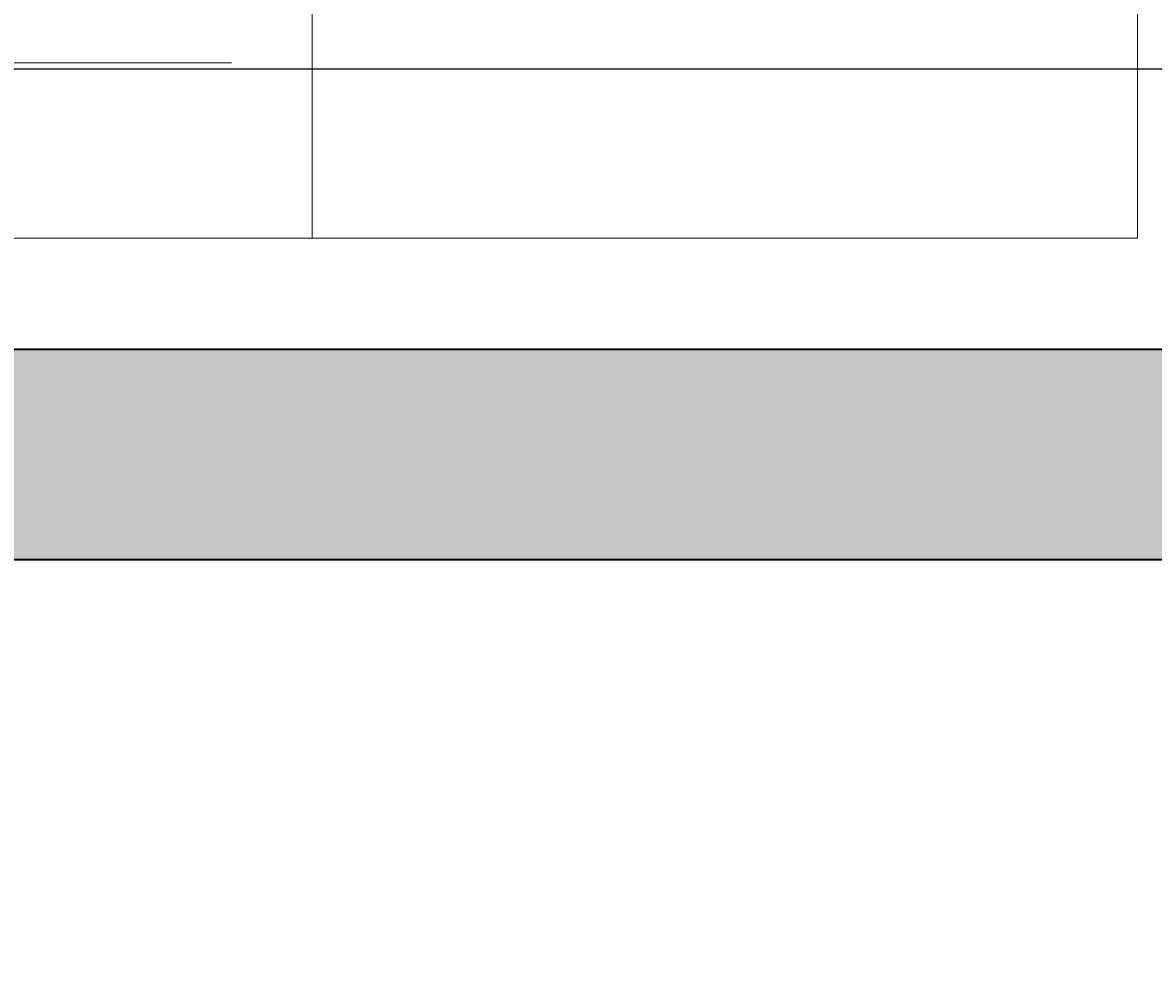
# Model space of a CAD drawing. Units: inches. Extents: x 1998 to 2588, y 1139 to 1977.
# Tile 16 of 134: x 2171 to 2195, y 1576 to 1596. Entities that reach past the tile are written whole.
import ezdxf

# ---------------------------------------------------------------- set-up
doc = ezdxf.new("R2010")
doc.units = ezdxf.units.IN
for name, color, linetype, lineweight in [('A-ANNO-DIMS', 2, 'Continuous', 18), ('A-FLOR-FIXT', 9, 'Continuous', 18), ('A-WALL-PATT', 252, 'Continuous', 13), ('WALL', 200, 'Continuous', 35)]:
    doc.layers.add(name, color=color, linetype=linetype, lineweight=lineweight)
doc.styles.get("Standard").update_dxf_attribs({"font": 'arial.ttf'})
doc.dimstyles.get("Standard").update_dxf_attribs({"dimtxt": 0.18, "dimasz": 0.18, "dimexe": 0.18, "dimexo": 0.0625, "dimgap": 0.09, "dimtad": 0, "dimtih": 1, "dimtoh": 1, "dimdec": 4, "dimzin": 0, "dimdsep": 46, "dimtxsty": 'Standard', "dimcen": 0.09, "dimadec": 0, "dimazin": 0, "dimtfac": 1, "dimtdec": 4, "dimtofl": 0, "dimtmove": 0, "dimatfit": 3, "dimfxl": 1, "dimtolj": 1, "dimtzin": 0, "dimarcsym": 0})

# ---------------------------------------------------------------- blocks, each defined once
blk = doc.blocks.new('SINK-WITH-DRAINBOARD')
for p, q in [((17.653, 0), (17.653, 19.174)), ((15.925, 17.391), (2.574, 17.391)), ((15.925, 15.023), (2.574, 15.023)), ((15.925, 12.848), (2.574, 12.848)), ((15.925, 10.383), (2.574, 10.383)), ((15.925, 8.143), (2.574, 8.143)), ((15.925, 5.899), (2.574, 5.899)), ((15.925, 3.752), (2.574, 3.752))]:
    blk.add_line(p, q)
blk.add_lwpolyline([(35.306, 19.174), (0, 19.174), (0, 0), (35.306, 0)], close=True)
blk.add_circle((25.956, 9.71), 1.353)
blk = doc.blocks.new('*D30')
at = {"layer": 'A-ANNO-DIMS', "color": 0, "lineweight": -2, "transparency": 16777216}
for p, q in [((2407.91, 1636.732), (1997.843, 1636.732)), ((1998.023, 1636.552), (1998.023, 1615.913)), ((1998.023, 1594.912), (1998.023, 1615.552)), ((2407.91, 1594.732), (1997.843, 1594.732))]:
    blk.add_line(p, q, dxfattribs=at)
at = {"layer": 'A-ANNO-DIMS', "color": 0, "transparency": 16777216}
for points in [[(1997.993, 1636.552), (1998.053, 1636.552), (1998.023, 1636.732)], [(1997.993, 1594.912), (1998.053, 1594.912), (1998.023, 1594.732)]]:
    blk.add_solid(points, dxfattribs=at)
at = {"layer": 'Defpoints', "color": 0, "transparency": 16777216}
for p in [(1998.023, 1636.732), (2407.973, 1636.732), (2407.973, 1594.732)]:
    blk.add_point(p, dxfattribs=at)
at = {"layer": 'A-ANNO-DIMS', "color": 0, "transparency": 16777216, "insert": (1998.023, 1615.732), "char_height": 0.18, "attachment_point": 5}
blk.add_mtext('\\A1;42', dxfattribs=at)
blk = doc.blocks.new('*D34')
at = {"layer": 'A-ANNO-DIMS', "color": 0, "lineweight": -2, "transparency": 16777216}
for p, q in [((2407.91, 1594.732), (1997.843, 1594.732)), ((1998.023, 1594.552), (1998.023, 1558.913)), ((1998.023, 1522.912), (1998.023, 1558.552)), ((2407.91, 1522.732), (1997.843, 1522.732))]:
    blk.add_line(p, q, dxfattribs=at)
at = {"layer": 'A-ANNO-DIMS', "color": 0, "transparency": 16777216}
for points in [[(1997.993, 1594.552), (1998.053, 1594.552), (1998.023, 1594.732)], [(1997.993, 1522.912), (1998.053, 1522.912), (1998.023, 1522.732)]]:
    blk.add_solid(points, dxfattribs=at)
at = {"layer": 'Defpoints', "color": 0, "transparency": 16777216}
for p in [(1998.023, 1594.732), (2407.973, 1594.732), (2407.973, 1522.732)]:
    blk.add_point(p, dxfattribs=at)
at = {"layer": 'A-ANNO-DIMS', "color": 0, "transparency": 16777216, "insert": (1998.023, 1558.732), "char_height": 0.18, "attachment_point": 5}
blk.add_mtext('\\A1;72', dxfattribs=at)

msp = doc.modelspace()

# ---------------------------------------------------------------- hatches: boundary and pattern name
at = {"layer": 'A-WALL-PATT'}
h = msp.add_hatch(color=256, dxfattribs=at)
h.dxf.hatch_style = 1
h.paths.add_polyline_path([(2222.9729, 1888.7324), (2099.4125, 1888.7324), (2099.4125, 1879.7324), (2222.9729, 1879.7324)])
h.paths.add_polyline_path([(2096.9729, 1868.3278), (2087.9729, 1868.3278), (2087.9729, 1775.637), (2096.9729, 1775.637)])
h.paths.add_polyline_path([(2227.4729, 1868.3278), (2222.9729, 1868.3278), (2222.9729, 1774.3318), (2227.4729, 1774.3318)])
h.paths.add_polyline_path([(2188.3019, 1759.7324), (2138.6074, 1759.7324), (2099.4125, 1759.7324), (2099.4125, 1755.2324), (2176.9729, 1755.2324), (2188.3019, 1755.2324)])
h.paths.add_polyline_path([(2087.9729, 1759.7324), (2059.4729, 1759.7324), (2059.4729, 1702.7324), (2087.9729, 1702.7324), (2087.9729, 1707.2324), (2063.9729, 1707.2324), (2063.9729, 1755.2324), (2087.9729, 1755.2324)])
h.paths.add_polyline_path([(2096.9729, 1755.2324), (2087.9729, 1755.2324), (2087.9729, 1707.2324), (2096.9729, 1707.2324)])
h.paths.add_polyline_path([(2187.0461, 1707.2324), (2105.9729, 1707.2324), (2096.9729, 1707.2324), (2087.9729, 1707.2324), (2087.9729, 1702.7324), (2105.9729, 1702.7324), (2114.9729, 1702.7324), (2187.0461, 1702.7324)])
h.paths.add_polyline_path([(2181.4729, 1719.2028), (2176.9729, 1719.2028), (2176.9729, 1707.2324), (2181.4729, 1707.2324)])
h.paths.add_polyline_path([(2216.0332, 1588.7324), (2114.9729, 1588.7324), (2105.9729, 1588.7324), (2105.9729, 1584.2324), (2216.0332, 1584.2324)])
h.paths.add_polyline_path([(2077.691, 1588.7324), (2061.4729, 1588.7324), (2061.4729, 1584.2324), (2077.691, 1584.2324)])
h.paths.add_polyline_path([(2105.9729, 1588.7324), (2098.0956, 1588.7324), (2098.0956, 1584.2324), (2105.9729, 1584.2324)])
h.paths.add_polyline_path([(2114.9729, 1596.2642), (2110.1012, 1596.2642), (2105.9729, 1596.2642), (2105.9729, 1588.7324), (2114.9729, 1588.7324)])
h.paths.add_polyline_path([(2114.9729, 1584.2324), (2105.9729, 1584.2324), (2105.9729, 1580.249), (2110.1012, 1580.249), (2114.9729, 1580.249)])
h.paths.add_polyline_path([(2114.9729, 1547.7716), (2110.1012, 1547.7716, -0.0318759), (2105.9729, 1548.035), (2105.9729, 1470.2324), (2108.3775, 1470.2324), (2108.3775, 1465.7324), (2186.2943, 1465.7324), (2186.2943, 1470.2324), (2114.9729, 1470.2324)])
h.paths.add_polyline_path([(2227.4729, 1584.2324), (2222.9729, 1584.2324), (2222.9729, 1486.137), (2227.4729, 1486.137)])
h.paths.add_polyline_path([(2295.4138, 1593.2324), (2227.4729, 1593.2324), (2227.4729, 1588.7324), (2295.4138, 1588.7324), (2295.4138, 1591.8729)])
h.paths.add_polyline_path([(2345.9729, 1627.1165), (2341.4729, 1627.1165), (2341.4729, 1593.2324), (2337.2869, 1593.2324), (2337.2869, 1591.8729), (2337.2869, 1588.7324), (2345.9729, 1588.7324)])
h.paths.add_polyline_path([(2291.9729, 1588.7324), (2287.4729, 1588.7324), (2287.4729, 1522.7324), (2291.9729, 1522.7324)])
h.paths.add_polyline_path([(2291.9729, 1522.7324), (2287.4729, 1522.7324), (2227.4729, 1522.7324), (2227.4729, 1518.2324), (2291.9729, 1518.2324)])
h.paths.add_polyline_path([(2295.7347, 1519.5919), (2295.7347, 1522.7324), (2291.9729, 1522.7324), (2291.9729, 1518.2324), (2295.7347, 1518.2324)])
h.paths.add_polyline_path([(2345.9729, 1522.7324), (2337.6078, 1522.7324), (2337.6078, 1519.5919), (2337.6078, 1518.2324), (2341.4729, 1518.2324), (2341.4729, 1488.5616), (2345.9729, 1488.5616)])
h.paths.add_polyline_path([(2345.9729, 1468.1569), (2341.4729, 1468.1569), (2341.4729, 1374.2324), (2227.4729, 1374.2324), (2227.4729, 1369.7324), (2345.9729, 1369.7324)])
h.paths.add_polyline_path([(2345.9729, 1369.7324), (2341.4729, 1369.7324), (2341.4729, 1362.2324), (2345.9729, 1362.2324)])
h.paths.add_polyline_path([(2345.9729, 1317.7324), (2345.9729, 1322.2324), (2341.4729, 1322.2324), (2341.4729, 1285.137), (2345.9729, 1285.137)], flags=17)
h.paths.add_polyline_path([(2356.2096, 1322.2324), (2345.9729, 1322.2324), (2345.9729, 1317.7324), (2356.2096, 1317.7324), (2356.2096, 1319.3088)], flags=17)
h.paths.add_polyline_path([(2393.9729, 1322.2324), (2375.6999, 1322.2324), (2375.6999, 1319.3088, -0.0202458), (2375.636, 1317.7324), (2393.9729, 1317.7324)], flags=17)
h.paths.add_polyline_path([(2398.4729, 1322.2324), (2393.9729, 1322.2324), (2393.9729, 1317.7324), (2393.9729, 1237.7324), (2345.9729, 1237.7324), (2345.9729, 1264.7324), (2341.4729, 1264.7324), (2341.4729, 1228.7324), (2393.9729, 1228.7324), (2482.7412, 1228.7324), (2482.7412, 1237.7324), (2398.4729, 1237.7324), (2398.4729, 1297.1029)])
h.paths.add_polyline_path([(2398.4729, 1362.2324), (2393.9729, 1362.2324), (2393.9729, 1357.7324), (2398.4729, 1357.7324)])
h.paths.add_polyline_path([(2345.9729, 1329.7549), (2341.4729, 1329.7549), (2341.4729, 1322.2324), (2345.9729, 1322.2324)])

# ---------------------------------------------------------------- linework, layer by layer
at = {"layer": 'WALL'}
for p, q in [((2216.0332, 1588.7324), (2114.9729, 1588.7324)), ((2227.4729, 1584.2324), (2105.9729, 1584.2324))]:
    msp.add_line(p, q, dxfattribs=at)

# ---------------------------------------------------------------- block references
at = {"layer": 'A-FLOR-FIXT'}
msp.add_blockref('SINK-WITH-DRAINBOARD', (2159.737, 1591.119), dxfattribs=at)

# ---------------------------------------------------------------- dimensions: what is measured, and where the dimension line sits
at = {"layer": 'A-ANNO-DIMS'}
for base, p1, p2, picture, middle in [((1998.0229, 1636.7324), (2407.9729, 1594.7324), (2407.9729, 1636.7324), '*D30', (1998.0229, 1615.7324)), ((1998.0229, 1594.7324), (2407.9729, 1522.7324), (2407.9729, 1594.7324), '*D34', (1998.0229, 1558.7324))]:
    dim = msp.add_linear_dim(base=base, p1=p1, p2=p2, angle=90, dimstyle='Standard', override={"dimdec": 0, "dimlfac": 1, "dimrnd": 0, "dimzin": 0, "dimdsep": 46, "dimlunit": 2}, dxfattribs=at)
    dim.commit()
    dim.dimension.update_dxf_attribs({"geometry": picture, "text_midpoint": middle})

doc.saveas('drawing.dxf')
